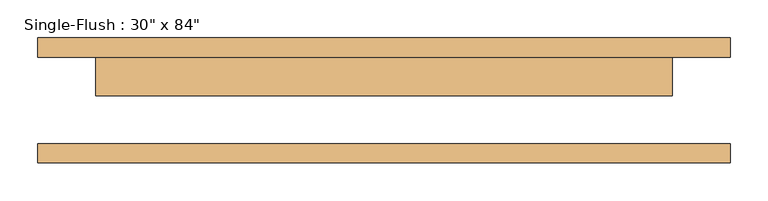
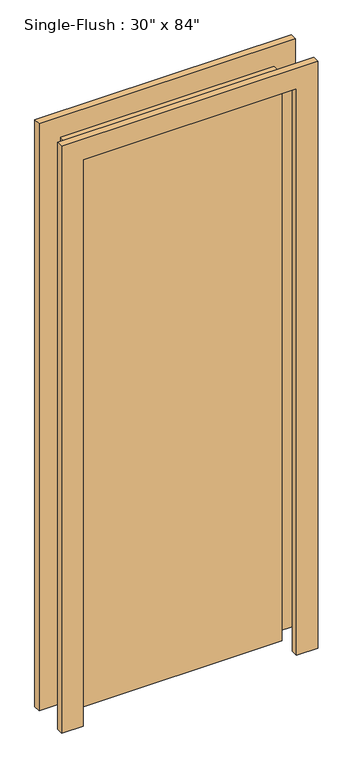
"""IFC4 building model written with IfcOpenShell, lengths in millimetres: door geometry."""

from ifc_helpers import new_model, si_unit, frame, origin, origin_with_axes, place, context, project, spatial, polyline, outline, extrude, source, transform, mapped, element, save


def door_214872d5(model_context):
    return source(origin(), model_context, "Body", "SweptSolid", [
        extrude(outline(polyline([(2209.8, -457.2), (0.0, -457.2), (0.0, -381.0), (2133.6, -381.0), (2133.6, 381.0), (0.0, 381.0), (0.0, 457.2), (2209.8, 457.2), (2209.8, -457.2)])), frame((0.0, 57.15, 0.0), z_axis=(0.0, 1.0, 0.0), x_axis=(0.0, 0.0, 1.0)), (0.0, 0.0, 1.0), 25.4),
        extrude(outline(polyline([(2209.8, 457.2), (2209.8, -457.2), (0.0, -457.2), (0.0, -381.0), (2133.6, -381.0), (2133.6, 381.0), (0.0, 381.0), (0.0, 457.2), (2209.8, 457.2)])), frame((0.0, -82.55, 0.0), z_axis=(0.0, 1.0, 0.0), x_axis=(0.0, 0.0, 1.0)), (0.0, 0.0, 1.0), 25.4),
        extrude(outline(polyline([(381.0, 6.35), (-381.0, 6.35), (-381.0, 57.15), (381.0, 57.15), (381.0, 6.35)])), origin_with_axes(), (0.0, 0.0, 1.0), 2133.6),
    ])


if __name__ == "__main__":
    model = new_model("IFC4")
    model_context = context("Model", 3, world=origin())
    ifc_project = project(units=[si_unit("LENGTHUNIT", "METRE", prefix="MILLI")], contexts=[model_context])
    site = spatial("IfcSite", under=ifc_project)
    building = spatial("IfcBuilding", under=site)
    placement = place(None, origin())
    door_shape = door_214872d5(model_context)
    element("IfcDoor", 1, ObjectType="Single-Flush : 30\" x 84\"", at=placement, inside=building, context=model_context, shape_type="MappedRepresentation", body=[
        mapped(door_shape, transform((0.0, 0.0, 0.0), x_axis=(1.0, 0.0, 0.0), y_axis=(0.0, 1.0, 0.0), z_axis=(0.0, 0.0, 1.0))),
    ])
    save(model, "model.ifc")

# Revit data of these elements
# Type "Single-Flush : 30\" x 84\""
#   Type Mark = "4"
#   Construction Type Id = "MDOOR"
#   Assembly Code = "C1020"
#   Analytic Construction = "Metal"
#   Thickness = 0.166667 ft
#   Heat Transfer Coefficient (U) = 0.651978 BTU/(h·ft²·°F)
#   Height = 7 ft
#   Trim Projection Ext = 0.083333 ft
#   Trim Projection Int = 0.083333 ft
#   Trim Width = 0.25 ft
#   Width = 2.5 ft
#   Define Thermal Properties by = 1
#   Define Thermal Properties by = 1
#   Door Material = Door - Panel
#   Frame Material = Door - Frame
#   Visual Light Transmittance = 0
#   Solar Heat Gain Coefficient = 0
#   Function = (empty or 0)
#   Wall Closure = (empty or 0)
# Element 1 (IfcDoor, "Single-Flush : 30\" x 84\"")
#   Materials on its faces: "Door - Frame", "Door - Panel"
# Materials
#   "Door - Panel": class "Wood", colour RGB 210 159 95, transparency 0, Cost = 0
#   "Door - Frame": colour RGB 118 70 51, transparency 0, Cost = 0
